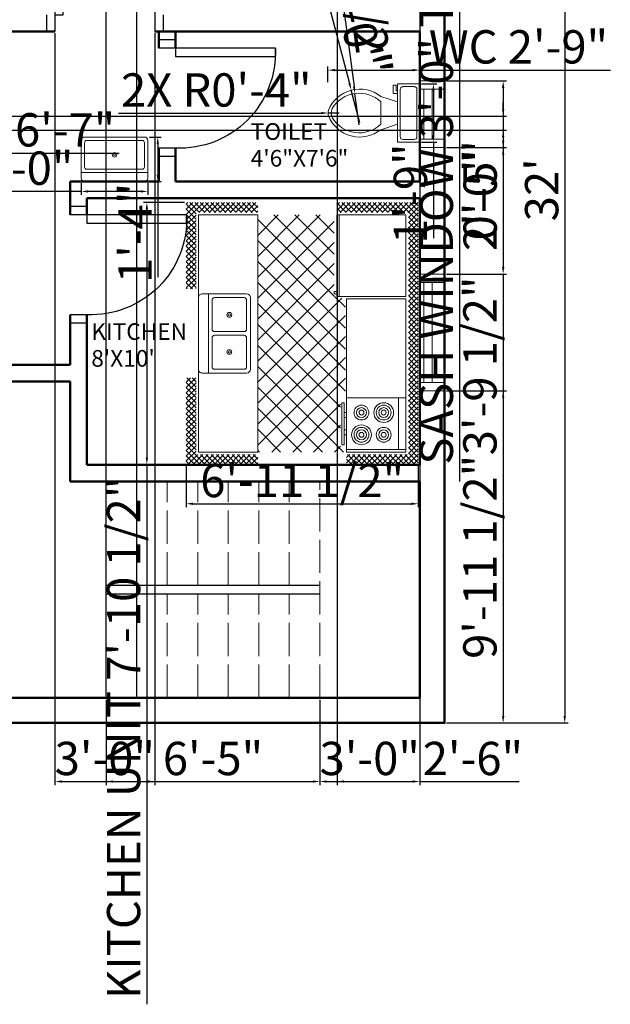
# Model space of a CAD drawing. Units: inches. Extents: x 3705 to 4206, y -1241 to -584.
# Tile 2 of 3: x 3921 to 4134, y -1241 to -886. Entities that reach past the tile are written whole.
import ezdxf

# ---------------------------------------------------------------- set-up
doc = ezdxf.new("R2010")
doc.units = ezdxf.units.IN
doc.linetypes.add('ACAD_ISO02W100', pattern=[15, 12, -3])
for name, color, linetype, lineweight in [('A-ANNO-DIMS', 2, 'Continuous', 18), ('A-AREA-IDEN', 7, 'Continuous', 25), ('A-DOOR', 3, 'Continuous', 25), ('A-FLOR-FIXT', 9, 'Continuous', 18), ('A-FLOR-STRS', 7, 'Continuous', 25), ('A-FLOR-STRS-HIDN', 8, 'ACAD_ISO02W100', 18), ('A-GLAZ', 4, 'Continuous', 18), ('A-WALL', 7, 'Continuous', 50)]:
    doc.layers.add(name, color=color, linetype=linetype, lineweight=lineweight)
doc.styles.get("Standard").update_dxf_attribs({"font": 'arial.ttf'})
doc.dimstyles.new('ISO-25', dxfattribs={"dimtxt": 12, "dimasz": 2.5, "dimexe": 1.25, "dimexo": 0.625, "dimtad": 1, "dimdec": 1, "dimlunit": 3, "dimtxsty": 'Standard', "dimcen": 2.5, "dimadec": 0, "dimazin": 0, "dimtfac": 1, "dimtdec": 1, "dimtmove": 0, "dimatfit": 3, "dimfxl": 1, "dimarcsym": 0})

# ---------------------------------------------------------------- blocks, each defined once
blk = doc.blocks.new('Toilet - top')
for p, q in [((9.5, -6), (9.5, -2)), ((-10, -8.5), (-8, -8.5)), ((-10, -9.5), (-10, -8.5)), ((-7, -9.5), (-10, -9.5)), ((-8, -8.5), (-8, -8)), ((-7, -8), (-7, -9.5)), ((-4, -8), (-6, -14)), ((4, -8), (6, -14)), ((4, -14), (-4, -14))]:
    blk.add_line(p, q)
blk.add_lwpolyline([(10.5, -8), (10.5, 0), (-10.5, 0), (-10.5, -8)], close=True)
for points in [[(-9.5, -2), (-9.5, -6)], [(8.5, -1), (-8.5, -1)], [(-8.5, -7), (8.5, -7)]]:
    blk.add_lwpolyline(points)
for centre, radius, start, end in [((-8.62, -1.88), 0.884, 81.8699, 188.1301), ((8.62, -1.88), 0.884, 351.8699, 98.1301), ((-8.62, -6.12), 0.884, 171.8699, 278.1301), ((8.62, -6.12), 0.884, 261.8699, 8.1301), ((3.52, -21.58), 12.17, 141.4691, 247.9714), ((4.2, -21.82), 11.33, 136.3677, 238.9468), ((-3.52, -21.58), 12.17, 292.0284, 38.5307), ((-4.2, -21.82), 11.33, 301.053, 43.6321), ((0, -27.88), 4, 245.7318, 294.2682), ((0, -29), 4, 254.8605, 285.1395)]:
    blk.add_arc(centre, radius, start, end)
blk = doc.blocks.new('Sink-single - 30 in top')
blk.add_line((-15, -3.999996), (15, -3.999996))
for points in [[(-13.5, 0), (13.5, 0)], [(-15, -18.499996), (-15, -1.5)], [(15, -1.5), (15, -18.499996)], [(-13.5, -17.499996), (-13.5, -6.499996)], [(-12.5, -5.499996), (12.5, -5.499996)], [(13.5, -6.499996), (13.5, -17.499996)], [(13.5, -19.999996), (-13.5, -19.999996)], [(12.5, -18.499996), (-12.5, -18.499996)]]:
    blk.add_lwpolyline(points)
for radius in [1, 0.5]:
    blk.add_circle((0, -11.999996), radius)
for centre, radius, start, end in [((-13.5, -1.5), 1.5, 90, 180), ((13.5, -1.5), 1.5, 0, 90), ((-12.5, -6.499996), 1, 90, 180), ((12.5, -6.499996), 1, 0, 90), ((-12.5, -17.499996), 1, 180, 270), ((12.5, -17.499996), 1, 270, 0), ((-13.5, -18.499996), 1.5, 180, 270), ((13.5, -18.499996), 1.5, 270, 0)]:
    blk.add_arc(centre, radius, start, end)
blk = doc.blocks.new('Kitchen Layout - 7 x 8 ft')
for p, q in [((-5, 81.32), (2.68, 89)), ((-5, 83.44), (0.56, 89)), ((-5, 85.56), (-1.56, 89)), ((-5, 87.68), (-3.68, 89)), ((-1, 84.97), (-5, 88.97)), ((1.09, 85), (-2.91, 89)), ((3.21, 85), (-0.79, 89)), ((0.81, 85), (4.81, 89)), ((5.34, 85), (1.34, 89)), ((2.93, 85), (6.93, 89)), ((7.46, 85), (3.46, 89)), ((5.05, 85), (9.05, 89)), ((9.58, 85), (5.58, 89)), ((7.17, 85), (11.17, 89)), ((11.7, 85), (7.7, 89)), ((9.29, 85), (13.29, 89)), ((13.82, 85), (9.82, 89)), ((11.41, 85), (15.41, 89)), ((15.94, 85), (11.94, 89)), ((13.53, 85), (17.53, 89)), ((18.06, 85), (14.06, 89)), ((15.65, 85), (19.65, 89)), ((20.18, 85), (16.18, 89)), ((17.78, 85), (21.78, 89)), ((22.31, 85), (18.31, 89)), ((19.9, 85), (23.9, 89)), ((24.43, 85), (20.43, 89)), ((22.02, 85), (26.02, 89)), ((26.55, 85), (22.55, 89)), ((24.14, 85), (28.14, 89)), ((28.67, 85), (24.67, 89)), ((26.26, 85), (30.26, 89)), ((30.79, 85), (26.79, 89)), ((28.38, 85), (32.38, 89)), ((32.91, 85), (28.91, 89)), ((30.5, 85), (34.5, 89)), ((35.03, 85), (31.03, 89)), ((32.63, 85), (36.63, 89)), ((37.16, 85), (33.16, 89)), ((34.75, 85), (38.75, 89)), ((39.28, 85), (35.28, 89)), ((36.87, 85), (40.87, 89)), ((41.4, 85), (37.4, 89)), ((38.99, 85), (42.99, 89)), ((43.52, 85), (39.52, 89)), ((41.11, 85), (45.11, 89)), ((45.64, 85), (41.64, 89)), ((43.23, 85), (47.23, 89)), ((47.76, 85), (43.76, 89)), ((45.35, 85), (49.35, 89)), ((49.88, 85), (45.88, 89)), ((47.47, 85), (51.47, 89)), ((52, 85), (48, 89)), ((49.6, 85), (53.6, 89)), ((54.13, 85), (50.13, 89)), ((51.72, 85), (55.72, 89)), ((56.25, 85), (52.25, 89)), ((53.84, 85), (57.84, 89)), ((58.37, 85), (54.37, 89)), ((55.96, 85), (59.96, 89)), ((60.49, 85), (56.49, 89)), ((58.08, 85), (62.08, 89)), ((62.61, 85), (58.61, 89)), ((60.2, 85), (64.2, 89)), ((64.73, 85), (60.73, 89)), ((62.32, 85), (66.32, 89)), ((66.85, 85), (62.85, 89)), ((64.45, 85), (68.45, 89)), ((68.97, 85), (64.97, 89)), ((66.57, 85), (70.57, 89)), ((71.1, 85), (67.1, 89)), ((68.69, 85), (72.69, 89)), ((73.22, 85), (69.22, 89)), ((70.81, 85), (74.81, 89)), ((75.34, 85), (71.34, 89)), ((72.93, 85), (76.93, 89)), ((77.46, 85), (73.46, 89)), ((75.05, 85), (79.05, 89)), ((79.58, 85), (75.58, 89)), ((77.17, 85), (81.17, 89)), ((81.7, 85), (77.7, 89)), ((79.29, 85), (83.29, 89)), ((83.82, 85), (79.82, 89)), ((81.42, 85), (85.42, 89)), ((85.95, 85), (81.95, 89)), ((83.54, 85), (87.54, 89)), ((88.07, 85), (84.07, 89)), ((85.66, 85), (89.66, 89)), ((90.19, 85), (86.19, 89)), ((87.78, 85), (91.78, 89)), ((92.31, 85), (88.31, 89)), ((89.9, 85), (93.9, 89)), ((94.43, 85), (90.43, 89)), ((92.02, 85), (96.02, 89)), ((96.55, 85), (92.55, 89)), ((94.14, 85), (98.14, 89)), ((101, 82.67), (94.67, 89)), ((96.27, 85), (100.27, 89)), ((101, 84.79), (96.79, 89)), ((101, 86.92), (98.92, 89)), ((-1, 82.85), (-5, 86.85)), ((-1, 80.73), (-5, 84.73)), ((34, 84), (96, 84)), ((34, 60), (34, 84)), ((96, 84), (96, 60)), ((97, 83.61), (101, 87.61)), ((97, 81.49), (101, 85.49)), ((101, 80.55), (97, 84.55)), ((-5, 79.19), (-1, 83.19)), ((-1, 78.61), (-5, 82.61)), ((-5, 77.07), (-1, 81.07)), ((-1, 76.49), (-5, 80.49)), ((74, 81), (95, 81)), ((97, 79.37), (101, 83.37)), ((101, 78.43), (97, 82.43)), ((97, 77.25), (101, 81.25)), ((101, 76.31), (97, 80.31)), ((-5, 74.95), (-1, 78.95)), ((-1, 74.36), (-5, 78.36)), ((-5, 72.83), (-1, 76.83)), ((-1, 72.24), (-5, 76.24)), ((97, 75.13), (101, 79.13)), ((101, 74.19), (97, 78.19)), ((97, 73.01), (101, 77.01)), ((101, 72.07), (97, 76.07)), ((-5, 70.71), (-1, 74.71)), ((-1, 70.12), (-5, 74.12)), ((-5, 68.59), (-1, 72.59)), ((-1, 68), (-5, 72)), ((97, 70.89), (101, 74.89)), ((101, 69.95), (97, 73.95)), ((97, 68.76), (101, 72.76)), ((101, 67.82), (97, 71.82)), ((-5, 66.47), (-1, 70.47)), ((-1, 65.88), (-5, 69.88)), ((-5, 64.35), (-1, 68.35)), ((-1, 63.76), (-5, 67.76)), ((97, 66.64), (101, 70.64)), ((101, 65.7), (97, 69.7)), ((97, 64.52), (101, 68.52)), ((-5, 62.22), (-1, 66.22)), ((-1, 61.64), (-5, 65.64)), ((-5, 60.1), (-1, 64.1)), ((101, 63.58), (97, 67.58)), ((97, 62.4), (101, 66.4)), ((101, 61.46), (97, 65.46)), ((97, 60.28), (101, 64.28)), ((-1, 59.52), (-5, 63.52)), ((-5, 57.98), (-1, 61.98)), ((-1, 57.39), (-5, 61.39)), ((-4.86, 56), (-1, 59.86)), ((96, 60), (34, 60)), ((80, 60), (80, 59)), ((82, 59), (82, 60)), ((87, 59), (87, 60)), ((89, 60), (89, 59)), ((100.34, 60), (97, 63.34)), ((98.22, 60), (97, 61.22)), ((98.84, 60), (101, 62.16)), ((100.96, 60), (101, 60.04)), ((-1.73, 56), (-5, 59.27)), ((-3.85, 56), (-5, 57.15)), ((-2.74, 56), (-1, 57.74)), ((0, 57), (33, 57)), ((10.4, 24), (45.9, 59.5)), ((18.88, 24), (54.38, 59.5)), ((27.37, 24), (62.87, 59.5)), ((31, 55), (31, 56)), ((32, 56), (32, 55)), ((33.03, 55.11), (37.41, 59.5)), ((67.71, 24), (33.68, 58.04)), ((35.85, 24), (71.35, 59.5)), ((76.2, 24), (40.7, 59.5)), ((44.34, 24), (77.84, 57.5)), ((84.68, 24), (49.18, 59.5)), ((52.82, 24), (86.32, 57.5)), ((93.17, 24), (57.67, 59.5)), ((61.31, 24), (96, 58.69)), ((96, 29.65), (66.15, 59.5)), ((96, 38.14), (76.64, 57.5)), ((96, 46.63), (85.13, 57.5)), ((96, 55.11), (93.57, 57.54)), ((0, 30.57), (24.43, 55)), ((0, 39.06), (15.94, 55)), ((0, 47.54), (7.46, 55)), ((1.91, 24), (32.91, 55)), ((33.77, 24), (2.77, 55)), ((42.26, 24), (11.26, 55)), ((50.74, 24), (19.74, 55)), ((59.23, 24), (28.23, 55)), ((32, 55), (31, 55)), ((25.29, 24), (0, 49.29)), ((69.79, 24), (96, 50.21)), ((16.8, 24), (0, 40.8)), ((78.28, 24), (96, 41.72)), ((8.32, 24), (0, 32.32)), ((86.76, 24), (96, 33.24)), ((-5, 21.92), (-2.92, 24)), ((-1, 21.33), (-3.67, 24)), ((-1, 23.45), (-1.55, 24)), ((0, 24), (96, 24)), ((0, 0), (0, 24)), ((95.25, 24), (96, 24.75)), ((96, 24), (96, 0)), ((97, 22.1), (98.9, 24)), ((97, 19.97), (101, 23.97)), ((101, 21.16), (98.16, 24)), ((101, 23.28), (100.28, 24)), ((-5, 19.8), (-1, 23.8)), ((-1, 19.21), (-5, 23.21)), ((-5, 17.68), (-1, 21.68)), ((-1, 17.09), (-5, 21.09)), ((101, 19.03), (97, 23.03)), ((97, 17.85), (101, 21.85)), ((101, 16.91), (97, 20.91)), ((-5, 15.55), (-1, 19.55)), ((-1, 14.97), (-5, 18.97)), ((-5, 13.43), (-1, 17.43)), ((-1, 12.85), (-5, 16.85)), ((47.25, 6.5), (47.25, 18.5)), ((48.75, 18.5), (48.75, 6.5)), ((97, 15.73), (101, 19.73)), ((101, 14.79), (97, 18.79)), ((97, 13.61), (101, 17.61)), ((101, 12.67), (97, 16.67)), ((-5, 11.31), (-1, 15.31)), ((-1, 10.73), (-5, 14.73)), ((-5, 9.19), (-1, 13.19)), ((-1, 8.6), (-5, 12.6)), ((97, 11.49), (101, 15.49)), ((101, 10.55), (97, 14.55)), ((97, 9.37), (101, 13.37)), ((101, 8.43), (97, 12.43)), ((-5, 7.07), (-1, 11.07)), ((-1, 6.48), (-5, 10.48)), ((-5, 4.95), (-1, 8.95)), ((-1, 4.36), (-5, 8.36)), ((97, 7.25), (101, 11.25)), ((101, 6.31), (97, 10.31)), ((97, 5.12), (101, 9.12)), ((101, 4.18), (97, 8.18)), ((-5, 2.83), (-1, 6.83)), ((-1, 2.24), (-5, 6.24)), ((-5, 0.71), (-1, 4.71)), ((-1, 0.12), (-5, 4.12)), ((64, 4), (32, 4)), ((97, 3), (101, 7)), ((101, 2.06), (97, 6.06)), ((97, 0.88), (101, 4.88)), ((-5, -1.42), (-1, 2.58)), ((2, -5), (-5, 2)), ((-5, -3.54), (-1, 0.46)), ((96, 0), (0, 0)), ((93.24, -5), (101, 2.76)), ((95.36, -5), (101, 0.64)), ((101, -0.06), (97, 3.94)), ((101, -2.18), (97, 1.82)), ((-0.12, -5), (-5, -0.12)), ((-2.25, -5), (-5, -2.25)), ((-4.34, -5), (-0.34, -1)), ((-2.22, -5), (1.78, -1)), ((-0.1, -5), (3.9, -1)), ((4.12, -5), (0.12, -1)), ((2.02, -5), (6.02, -1)), ((6.24, -5), (2.24, -1)), ((4.14, -5), (8.14, -1)), ((8.36, -5), (4.36, -1)), ((6.27, -5), (10.27, -1)), ((10.48, -5), (6.48, -1)), ((8.39, -5), (12.39, -1)), ((12.6, -5), (8.6, -1)), ((10.51, -5), (14.51, -1)), ((14.73, -5), (10.73, -1)), ((12.63, -5), (16.63, -1)), ((16.85, -5), (12.85, -1)), ((14.75, -5), (18.75, -1)), ((18.97, -5), (14.97, -1)), ((16.87, -5), (20.87, -1)), ((21.09, -5), (17.09, -1)), ((18.99, -5), (22.99, -1)), ((23.21, -5), (19.21, -1)), ((21.11, -5), (25.11, -1)), ((25.33, -5), (21.33, -1)), ((23.24, -5), (27.24, -1)), ((27.45, -5), (23.45, -1)), ((25.36, -5), (29.36, -1)), ((29.57, -5), (25.57, -1)), ((27.48, -5), (30, -2.48)), ((30, -3.3), (27.7, -1)), ((30, -1.18), (29.82, -1)), ((66, -2.54), (67.54, -1)), ((66, -4.66), (69.66, -1)), ((69.88, -5), (66, -1.12)), ((67.76, -5), (66, -3.24)), ((67.78, -5), (71.78, -1)), ((72, -5), (68, -1)), ((69.9, -5), (73.9, -1)), ((74.12, -5), (70.12, -1)), ((72.03, -5), (76.03, -1)), ((76.24, -5), (72.24, -1)), ((74.15, -5), (78.15, -1)), ((78.36, -5), (74.36, -1)), ((76.27, -5), (80.27, -1)), ((80.49, -5), (76.49, -1)), ((78.39, -5), (82.39, -1)), ((82.61, -5), (78.61, -1)), ((80.51, -5), (84.51, -1)), ((84.73, -5), (80.73, -1)), ((82.63, -5), (86.63, -1)), ((86.85, -5), (82.85, -1)), ((84.75, -5), (88.75, -1)), ((88.97, -5), (84.97, -1)), ((86.88, -5), (90.88, -1)), ((91.09, -5), (87.09, -1)), ((89, -5), (93, -1)), ((93.21, -5), (89.21, -1)), ((91.12, -5), (95.12, -1)), ((95.34, -5), (91.34, -1)), ((97.46, -5), (93.46, -1)), ((99.58, -5), (95.58, -1)), ((101, -4.3), (97, -0.3)), ((97.48, -5), (101, -1.48)), ((99.6, -5), (101, -3.6)), ((-4.37, -5), (-5, -4.37)), ((29.6, -5), (30, -4.6))]:
    blk.add_line(p, q)
for points in [[(0, 56), (0, 84), (33, 84), (33, 56)], [(74, 60), (74, 84), (95, 84), (95, 60)], [(76, 58), (76, 59), (93, 59), (93, 58)]]:
    blk.add_lwpolyline(points, close=True)
for points in [[(33.5, 21), (62.5, 21)], [(32, 1.5), (32, 19.5)], [(33.5, 6.5), (33.5, 18.5)], [(34.5, 19.5), (46.25, 19.5)], [(49.75, 19.5), (61.5, 19.5)], [(62.5, 18.5), (62.5, 6.5)], [(64, 19.5), (64, 1.5)], [(46.25, 5.5), (34.5, 5.5)], [(61.5, 5.5), (49.75, 5.5)], [(62.5, 0), (33.5, 0)]]:
    blk.add_lwpolyline(points)
for centre, radius in [((80, 75), 4), ((80, 75), 3), ((80, 75), 2), ((80, 75), 1), ((89, 75), 3), ((89, 75), 2), ((89, 75), 1), ((80, 66), 3), ((80, 66), 2), ((89, 66), 4), ((89, 66), 3), ((89, 66), 2), ((80, 66), 1), ((89, 66), 1), ((40.5, 12.5), 1), ((40.5, 12.5), 0.5), ((55.5, 12.5), 1), ((55.5, 12.5), 0.5)]:
    blk.add_circle(centre, radius)
for centre, radius, start, end in [((33.5, 19.5), 1.5, 90, 180), ((62.5, 19.5), 1.5, 0, 90), ((34.5, 18.5), 1, 90, 180), ((46.25, 18.5), 1, 0, 90), ((49.75, 18.5), 1, 90, 180), ((61.5, 18.5), 1, 0, 90), ((34.5, 6.5), 1, 180, 270), ((46.25, 6.5), 1, 270, 0), ((49.75, 6.5), 1, 180, 270), ((61.5, 6.5), 1, 270, 0), ((33.5, 1.5), 1.5, 180, 270), ((62.5, 1.5), 1.5, 270, 0)]:
    blk.add_arc(centre, radius, start, end)
blk = doc.blocks.new('*D12')
at = {"layer": 'A-ANNO-DIMS', "color": 0, "lineweight": -2, "transparency": 16777216}
for p, q in [((4074.7, -755.75), (4118.62, -755.75)), ((4117.37, -758.25), (4117.37, -1137.25)), ((4074.7, -1139.75), (4118.62, -1139.75))]:
    blk.add_line(p, q, dxfattribs=at)
at = {"layer": 'A-ANNO-DIMS', "color": 0, "transparency": 16777216}
for points in [[(4116.95, -758.25), (4117.78, -758.25), (4117.37, -755.75)], [(4116.95, -1137.25), (4117.78, -1137.25), (4117.37, -1139.75)]]:
    blk.add_solid(points, dxfattribs=at)
at = {"layer": 'Defpoints', "color": 0, "transparency": 16777216}
for p in [(4074.08, -755.75), (4074.08, -1139.75), (4117.37, -1139.75)]:
    blk.add_point(p, dxfattribs=at)
at = {"layer": 'A-ANNO-DIMS', "color": 0, "transparency": 16777216, "insert": (4110.61, -947.75), "char_height": 12, "attachment_point": 5, "rotation": 90}
blk.add_mtext("32'", dxfattribs=at)
blk = doc.blocks.new('DOOR-SINGLE-36IN')
for p, q in [((0, 6), (0, 0)), ((3, 6), (3, 0)), ((39, 6), (39, 0)), ((42, 6), (42, 0))]:
    blk.add_line(p, q)
blk.add_lwpolyline([(39, 6), (36, 6), (36, 42), (39, 42)], close=True)
blk.add_arc((37.5, 7.5), 34.53, 87.5104, 182.4896)
blk = doc.blocks.new('WIN-SASH-36IN')
for p, q in [((0, 9), (0, 0)), ((36, 0), (36, 9)), ((0, 4.5), (36, 4.5)), ((0, 1.5), (36, 1.5)), ((0, 1.5), (36, 1.5))]:
    blk.add_line(p, q)
blk = doc.blocks.new('*D15')
at = {"layer": 'A-ANNO-DIMS', "color": 0, "lineweight": -2, "transparency": 16777216}
for p, q in [((4074.7, -811.42), (4080.73, -811.42)), ((4079.48, -813.92), (4079.48, -844.92)), ((4074.7, -847.42), (4080.73, -847.42)), ((4079.48, -847.42), (4079.48, -1052.78))]:
    blk.add_line(p, q, dxfattribs=at)
at = {"layer": 'A-ANNO-DIMS', "color": 0, "transparency": 16777216}
for points in [[(4079.06, -813.92), (4079.9, -813.92), (4079.48, -811.42)], [(4079.06, -844.92), (4079.9, -844.92), (4079.48, -847.42)]]:
    blk.add_solid(points, dxfattribs=at)
at = {"layer": 'Defpoints', "color": 0, "transparency": 16777216}
for p in [(4074.08, -811.42), (4074.08, -847.42), (4079.48, -847.42)]:
    blk.add_point(p, dxfattribs=at)
at = {"layer": 'A-ANNO-DIMS', "color": 0, "transparency": 16777216, "insert": (4072.64, -951.35), "char_height": 12, "attachment_point": 5, "rotation": 90}
blk.add_mtext('SASH WINDOW 3\'-0" TYP.', dxfattribs=at)
blk = doc.blocks.new('*D25')
at = {"layer": 'A-ANNO-DIMS', "color": 0, "lineweight": -2, "transparency": 16777216}
for p, q in [((3791.85, -923.33), (3791.85, -935.8)), ((3870.81, -923.33), (3870.81, -935.8)), ((3794.35, -934.55), (3868.31, -934.55)), ((3870.81, -934.55), (3956.7, -934.55))]:
    blk.add_line(p, q, dxfattribs=at)
at = {"layer": 'A-ANNO-DIMS', "color": 0, "transparency": 16777216}
for points in [[(3794.35, -934.13), (3794.35, -934.97), (3791.85, -934.55)], [(3868.31, -934.13), (3868.31, -934.97), (3870.81, -934.55)]]:
    blk.add_solid(points, dxfattribs=at)
at = {"layer": 'Defpoints', "color": 0, "transparency": 16777216}
for p in [(3791.85, -922.71), (3870.81, -922.71), (3870.81, -934.55)]:
    blk.add_point(p, dxfattribs=at)
at = {"layer": 'A-ANNO-DIMS', "color": 0, "transparency": 16777216, "insert": (3915, -927.72), "char_height": 12, "attachment_point": 5}
blk.add_mtext('SOFA 6\'-7"', dxfattribs=at)
blk = doc.blocks.new('*D29')
at = {"layer": 'A-ANNO-DIMS', "color": 0, "lineweight": -2, "transparency": 16777216}
for p, q in [((4032.03, -908.99), (4032.03, -903.41)), ((4065.08, -908.99), (4065.08, -903.41)), ((4034.53, -904.66), (4062.58, -904.66)), ((4065.08, -904.66), (4133.81, -904.66))]:
    blk.add_line(p, q, dxfattribs=at)
at = {"layer": 'A-ANNO-DIMS', "color": 0, "transparency": 16777216}
for points in [[(4034.53, -904.24), (4034.53, -905.07), (4032.03, -904.66)], [(4062.58, -904.24), (4062.58, -905.07), (4065.08, -904.66)]]:
    blk.add_solid(points, dxfattribs=at)
at = {"layer": 'Defpoints', "color": 0, "transparency": 16777216}
for p in [(4065.08, -904.66), (4032.03, -909.61), (4065.08, -909.61)]:
    blk.add_point(p, dxfattribs=at)
at = {"layer": 'A-ANNO-DIMS', "color": 0, "transparency": 16777216, "insert": (4100.69, -897.83), "char_height": 12, "attachment_point": 5}
blk.add_mtext('WC 2\'-9"', dxfattribs=at)
blk = doc.blocks.new('*D30')
at = {"layer": 'A-ANNO-DIMS', "color": 0, "lineweight": -2, "transparency": 16777216}
for p, q in [((4065.7, -909.61), (4071.29, -909.61)), ((4070.04, -912.11), (4070.04, -928.11)), ((4065.7, -930.61), (4071.29, -930.61)), ((4070.04, -930.61), (4070.04, -965.13))]:
    blk.add_line(p, q, dxfattribs=at)
at = {"layer": 'A-ANNO-DIMS', "color": 0, "transparency": 16777216}
for points in [[(4069.62, -912.11), (4070.45, -912.11), (4070.04, -909.61)], [(4069.62, -928.11), (4070.45, -928.11), (4070.04, -930.61)]]:
    blk.add_solid(points, dxfattribs=at)
at = {"layer": 'Defpoints', "color": 0, "transparency": 16777216}
for p in [(4065.08, -909.61), (4065.08, -930.61), (4070.04, -930.61)]:
    blk.add_point(p, dxfattribs=at)
at = {"layer": 'A-ANNO-DIMS', "color": 0, "transparency": 16777216, "insert": (4063.28, -949.12), "char_height": 12, "attachment_point": 5, "rotation": 90}
blk.add_mtext('1\'-9"', dxfattribs=at)
blk = doc.blocks.new('*D31')
at = {"layer": 'A-ANNO-DIMS', "color": 0, "lineweight": -2, "transparency": 16777216}
for p, q in [((3943.08, -945.37), (3943.08, -949.6)), ((3967.08, -945.37), (3967.08, -949.6)), ((3943.08, -948.35), (3853, -948.35)), ((3964.58, -948.35), (3945.58, -948.35))]:
    blk.add_line(p, q, dxfattribs=at)
at = {"layer": 'A-ANNO-DIMS', "color": 0, "transparency": 16777216}
for points in [[(3945.58, -947.93), (3945.58, -948.76), (3943.08, -948.35)], [(3964.58, -947.93), (3964.58, -948.76), (3967.08, -948.35)]]:
    blk.add_solid(points, dxfattribs=at)
at = {"layer": 'Defpoints', "color": 0, "transparency": 16777216}
for p in [(3943.08, -944.75), (3967.08, -944.75), (3943.08, -948.35)]:
    blk.add_point(p, dxfattribs=at)
at = {"layer": 'A-ANNO-DIMS', "color": 0, "transparency": 16777216, "insert": (3896.79, -941.52), "char_height": 12, "attachment_point": 5}
blk.add_mtext('BASIN 2\'-0"', dxfattribs=at)
blk = doc.blocks.new('*D32')
at = {"layer": 'A-ANNO-DIMS', "color": 0, "lineweight": -2, "transparency": 16777216}
for p, q in [((3967.7, -928.75), (3971.93, -928.75)), ((3970.68, -931.25), (3970.68, -942.25)), ((3967.7, -944.75), (3971.93, -944.75)), ((3970.68, -944.75), (3970.68, -979.27))]:
    blk.add_line(p, q, dxfattribs=at)
at = {"layer": 'A-ANNO-DIMS', "color": 0, "transparency": 16777216}
for points in [[(3970.26, -931.25), (3971.1, -931.25), (3970.68, -928.75)], [(3970.26, -942.25), (3971.1, -942.25), (3970.68, -944.75)]]:
    blk.add_solid(points, dxfattribs=at)
at = {"layer": 'Defpoints', "color": 0, "transparency": 16777216}
for p in [(3967.08, -928.75), (3967.08, -944.75), (3970.68, -944.75)]:
    blk.add_point(p, dxfattribs=at)
at = {"layer": 'A-ANNO-DIMS', "color": 0, "transparency": 16777216, "insert": (3964.03, -963.26), "char_height": 12, "attachment_point": 5, "rotation": 90}
blk.add_mtext('1\'-4"', dxfattribs=at)
blk = doc.blocks.new('*D33')
at = {"layer": 'A-ANNO-DIMS', "color": 0, "lineweight": -2, "transparency": 16777216}
for p, q in [((3980.27, -952.31), (3965.49, -952.31)), ((3966.74, -954.81), (3966.74, -1044.17)), ((3980.27, -1046.67), (3965.49, -1046.67)), ((3966.74, -1046.67), (3966.74, -1241.08))]:
    blk.add_line(p, q, dxfattribs=at)
at = {"layer": 'A-ANNO-DIMS', "color": 0, "transparency": 16777216}
for points in [[(3966.32, -954.81), (3967.16, -954.81), (3966.74, -952.31)], [(3966.32, -1044.17), (3967.16, -1044.17), (3966.74, -1046.67)]]:
    blk.add_solid(points, dxfattribs=at)
at = {"layer": 'Defpoints', "color": 0, "transparency": 16777216}
for p in [(3980.9, -952.31), (3966.74, -1046.67), (3980.9, -1046.67)]:
    blk.add_point(p, dxfattribs=at)
at = {"layer": 'A-ANNO-DIMS', "color": 0, "transparency": 16777216, "insert": (3959.91, -1145.12), "char_height": 12, "attachment_point": 5, "rotation": 90}
blk.add_mtext('KITCHEN UNIT 7\'-10 1/2"', dxfattribs=at)
blk = doc.blocks.new('*D34')
at = {"layer": 'A-ANNO-DIMS', "color": 0, "lineweight": -2, "transparency": 16777216}
for p, q in [((3980.9, -1047.29), (3980.9, -1062.07)), ((4064.57, -1047.29), (4064.57, -1062.07)), ((3983.4, -1060.82), (4062.07, -1060.82))]:
    blk.add_line(p, q, dxfattribs=at)
at = {"layer": 'A-ANNO-DIMS', "color": 0, "transparency": 16777216}
for points in [[(3983.4, -1060.4), (3983.4, -1061.24), (3980.9, -1060.82)], [(4062.07, -1060.4), (4062.07, -1061.24), (4064.57, -1060.82)]]:
    blk.add_solid(points, dxfattribs=at)
at = {"layer": 'Defpoints', "color": 0, "transparency": 16777216}
for p in [(3980.9, -1046.67), (4064.57, -1046.67), (4064.57, -1060.82)]:
    blk.add_point(p, dxfattribs=at)
at = {"layer": 'A-ANNO-DIMS', "color": 0, "transparency": 16777216, "insert": (4022.73, -1053.99), "char_height": 12, "attachment_point": 5}
blk.add_mtext('6\'-11 1/2"', dxfattribs=at)
blk = doc.blocks.new('*D40')
at = {"layer": 'A-ANNO-DIMS', "color": 0, "lineweight": -2, "transparency": 16777216}
for p, q in [((4074.7, -1020.11), (4096.43, -1020.11)), ((4095.18, -1022.61), (4095.18, -1137.25)), ((4074.7, -1139.75), (4096.43, -1139.75))]:
    blk.add_line(p, q, dxfattribs=at)
at = {"layer": 'A-ANNO-DIMS', "color": 0, "transparency": 16777216}
for points in [[(4094.76, -1022.61), (4095.6, -1022.61), (4095.18, -1020.11)], [(4094.76, -1137.25), (4095.6, -1137.25), (4095.18, -1139.75)]]:
    blk.add_solid(points, dxfattribs=at)
at = {"layer": 'Defpoints', "color": 0, "transparency": 16777216}
for p in [(4074.08, -1020.11), (4074.08, -1139.75), (4095.18, -1139.75)]:
    blk.add_point(p, dxfattribs=at)
at = {"layer": 'A-ANNO-DIMS', "color": 0, "transparency": 16777216, "insert": (4088.35, -1079.93), "char_height": 12, "attachment_point": 5, "rotation": 90}
blk.add_mtext('9\'-11 1/2"', dxfattribs=at)
blk = doc.blocks.new('*D41')
at = {"layer": 'A-ANNO-DIMS', "color": 0, "lineweight": -2, "transparency": 16777216}
for p, q in [((4074.7, -932.56), (4096.43, -932.56)), ((4095.18, -935.06), (4095.18, -975.61)), ((4074.7, -978.11), (4096.43, -978.11)), ((4095.18, -978.11), (4095.18, -1041.72))]:
    blk.add_line(p, q, dxfattribs=at)
at = {"layer": 'A-ANNO-DIMS', "color": 0, "transparency": 16777216}
for points in [[(4094.76, -935.06), (4095.6, -935.06), (4095.18, -932.56)], [(4094.76, -975.61), (4095.6, -975.61), (4095.18, -978.11)]]:
    blk.add_solid(points, dxfattribs=at)
at = {"layer": 'Defpoints', "color": 0, "transparency": 16777216}
for p in [(4074.08, -932.56), (4074.08, -978.11), (4095.18, -978.11)]:
    blk.add_point(p, dxfattribs=at)
at = {"layer": 'A-ANNO-DIMS', "color": 0, "transparency": 16777216, "insert": (4088.35, -1011.17), "char_height": 12, "attachment_point": 5, "rotation": 90}
blk.add_mtext('3\'-9 1/2"', dxfattribs=at)
blk = doc.blocks.new('*D42')
at = {"layer": 'A-ANNO-DIMS', "color": 0, "lineweight": -2, "transparency": 16777216}
for p, q in [((4074.7, -908.56), (4096.43, -908.56)), ((4095.18, -911.06), (4095.18, -930.06)), ((4074.7, -932.56), (4096.43, -932.56)), ((4095.18, -932.56), (4095.18, -968.41))]:
    blk.add_line(p, q, dxfattribs=at)
at = {"layer": 'A-ANNO-DIMS', "color": 0, "transparency": 16777216}
for points in [[(4094.76, -911.06), (4095.6, -911.06), (4095.18, -908.56)], [(4094.76, -930.06), (4095.6, -930.06), (4095.18, -932.56)]]:
    blk.add_solid(points, dxfattribs=at)
at = {"layer": 'Defpoints', "color": 0, "transparency": 16777216}
for p in [(4074.08, -908.56), (4074.08, -932.56), (4095.18, -932.56)]:
    blk.add_point(p, dxfattribs=at)
at = {"layer": 'A-ANNO-DIMS', "color": 0, "transparency": 16777216, "insert": (4088.43, -951.74), "char_height": 12, "attachment_point": 5, "rotation": 90}
blk.add_mtext('2\'-0"', dxfattribs=at)
blk = doc.blocks.new('*D45')
at = {"layer": 'A-ANNO-DIMS', "color": 0, "lineweight": -2, "transparency": 16777216}
for p, q in [((3952.08, -1131.37), (3952.08, -1162.1)), ((4029.08, -1131.37), (4029.08, -1162.1)), ((3954.58, -1160.85), (4026.58, -1160.85))]:
    blk.add_line(p, q, dxfattribs=at)
at = {"layer": 'A-ANNO-DIMS', "color": 0, "transparency": 16777216}
for points in [[(3954.58, -1160.43), (3954.58, -1161.26), (3952.08, -1160.85)], [(4026.58, -1160.43), (4026.58, -1161.26), (4029.08, -1160.85)]]:
    blk.add_solid(points, dxfattribs=at)
at = {"layer": 'Defpoints', "color": 0, "transparency": 16777216}
for p in [(3952.08, -1130.75), (4029.08, -1130.75), (4029.08, -1160.85)]:
    blk.add_point(p, dxfattribs=at)
at = {"layer": 'A-ANNO-DIMS', "color": 0, "transparency": 16777216, "insert": (3990.58, -1154.1), "char_height": 12, "attachment_point": 5}
blk.add_mtext('6\'-5"', dxfattribs=at)
blk = doc.blocks.new('*D46')
at = {"layer": 'A-ANNO-DIMS', "color": 0, "lineweight": -2, "transparency": 16777216}
for p, q in [((4029.08, -1131.37), (4029.08, -1162.1)), ((4065.08, -1131.37), (4065.08, -1162.1)), ((4031.58, -1160.85), (4062.58, -1160.85))]:
    blk.add_line(p, q, dxfattribs=at)
at = {"layer": 'A-ANNO-DIMS', "color": 0, "transparency": 16777216}
for points in [[(4031.58, -1160.43), (4031.58, -1161.26), (4029.08, -1160.85)], [(4062.58, -1160.43), (4062.58, -1161.26), (4065.08, -1160.85)]]:
    blk.add_solid(points, dxfattribs=at)
at = {"layer": 'Defpoints', "color": 0, "transparency": 16777216}
for p in [(4029.08, -1130.75), (4065.08, -1130.75), (4065.08, -1160.85)]:
    blk.add_point(p, dxfattribs=at)
at = {"layer": 'A-ANNO-DIMS', "color": 0, "transparency": 16777216, "insert": (4047.08, -1154.09), "char_height": 12, "attachment_point": 5}
blk.add_mtext('3\'-0"', dxfattribs=at)
blk = doc.blocks.new('*D51')
at = {"layer": 'A-ANNO-DIMS', "color": 0, "lineweight": -2, "transparency": 16777216}
for p, q in [((3933.58, -891.37), (3933.58, -1162.1)), ((3969.58, -891.37), (3969.58, -1162.1)), ((3936.08, -1160.85), (3967.08, -1160.85))]:
    blk.add_line(p, q, dxfattribs=at)
at = {"layer": 'A-ANNO-DIMS', "color": 0, "transparency": 16777216}
for points in [[(3936.08, -1160.43), (3936.08, -1161.26), (3933.58, -1160.85)], [(3967.08, -1160.43), (3967.08, -1161.26), (3969.58, -1160.85)]]:
    blk.add_solid(points, dxfattribs=at)
at = {"layer": 'Defpoints', "color": 0, "transparency": 16777216}
for p in [(3933.58, -890.75), (3969.58, -890.75), (3969.58, -1160.85)]:
    blk.add_point(p, dxfattribs=at)
at = {"layer": 'A-ANNO-DIMS', "color": 0, "transparency": 16777216, "insert": (3951.58, -1154.09), "char_height": 12, "attachment_point": 5}
blk.add_mtext('3\'-0"', dxfattribs=at)
blk = doc.blocks.new('*D53')
at = {"layer": 'A-ANNO-DIMS', "color": 0, "lineweight": -2, "transparency": 16777216}
for p, q in [((3952.08, -1130.12), (3952.08, -733.4)), ((3963.08, -1130.12), (3963.08, -733.4)), ((3954.58, -734.65), (3960.58, -734.65)), ((3963.08, -734.65), (4008.05, -734.65))]:
    blk.add_line(p, q, dxfattribs=at)
at = {"layer": 'A-ANNO-DIMS', "color": 0, "transparency": 16777216}
for points in [[(3954.58, -734.23), (3954.58, -735.06), (3952.08, -734.65)], [(3960.58, -734.23), (3960.58, -735.06), (3963.08, -734.65)]]:
    blk.add_solid(points, dxfattribs=at)
at = {"layer": 'Defpoints', "color": 0, "transparency": 16777216}
for p in [(3963.08, -734.65), (3952.08, -1130.75), (3963.08, -1130.75)]:
    blk.add_point(p, dxfattribs=at)
at = {"layer": 'A-ANNO-DIMS', "color": 0, "transparency": 16777216, "insert": (3986.82, -727.9), "char_height": 12, "attachment_point": 5}
blk.add_mtext('0\'-11"', dxfattribs=at)
blk = doc.blocks.new('*D55')
at = {"layer": 'A-ANNO-DIMS', "color": 0, "lineweight": -2, "transparency": 16777216}
for p, q in [((4035.32, -845.43), (4035.32, -1162.1)), ((4065.08, -851.05), (4065.08, -1162.1)), ((4037.82, -1160.85), (4062.58, -1160.85)), ((4065.08, -1160.85), (4100.93, -1160.85))]:
    blk.add_line(p, q, dxfattribs=at)
at = {"layer": 'A-ANNO-DIMS', "color": 0, "transparency": 16777216}
for points in [[(4037.82, -1160.43), (4037.82, -1161.26), (4035.32, -1160.85)], [(4062.58, -1160.43), (4062.58, -1161.26), (4065.08, -1160.85)]]:
    blk.add_solid(points, dxfattribs=at)
at = {"layer": 'Defpoints', "color": 0, "transparency": 16777216}
for p in [(4035.32, -844.8), (4065.08, -850.42), (4065.08, -1160.85)]:
    blk.add_point(p, dxfattribs=at)
at = {"layer": 'A-ANNO-DIMS', "color": 0, "transparency": 16777216, "insert": (4084.26, -1154.1), "char_height": 12, "attachment_point": 5}
blk.add_mtext('2\'-6"', dxfattribs=at)
blk = doc.blocks.new('*D59')
at = {"layer": 'A-ANNO-DIMS', "color": 0, "lineweight": -2, "transparency": 16777216}
for p, q in [((4095.18, -918.74), (4095.18, -916.24)), ((3865.79, -921.24), (4096.43, -921.24)), ((4095.18, -921.24), (4095.18, -926.33)), ((3837.22, -926.33), (4096.43, -926.33)), ((4095.18, -928.83), (4095.18, -964.48))]:
    blk.add_line(p, q, dxfattribs=at)
at = {"layer": 'A-ANNO-DIMS', "color": 0, "transparency": 16777216}
for points in [[(4094.76, -918.74), (4095.6, -918.74), (4095.18, -921.24)], [(4094.76, -928.83), (4095.6, -928.83), (4095.18, -926.33)]]:
    blk.add_solid(points, dxfattribs=at)
at = {"layer": 'Defpoints', "color": 0, "transparency": 16777216}
for p in [(3865.17, -921.24), (3836.59, -926.33), (4095.18, -926.33)]:
    blk.add_point(p, dxfattribs=at)
at = {"layer": 'A-ANNO-DIMS', "color": 0, "transparency": 16777216, "insert": (4088.43, -947.91), "char_height": 12, "attachment_point": 5, "rotation": 90}
blk.add_mtext('0\'-5"', dxfattribs=at)
blk = doc.blocks.new('*D66')
at = {"layer": 'A-ANNO-DIMS', "color": 0, "lineweight": -2, "transparency": 16777216}
for p, q in [((4021.19, -838.72), (4039.77, -909.45)), ((4043.5, -923.63), (4040.41, -911.86))]:
    blk.add_line(p, q, dxfattribs=at)
at = {"layer": 'A-ANNO-DIMS', "color": 0, "transparency": 16777216}
blk.add_solid([(4040.17, -909.34), (4039.37, -909.55), (4040.41, -911.86)], dxfattribs=at)
at = {"layer": 'Defpoints', "color": 0, "transparency": 16777216}
for p in [(4040.41, -911.86), (4043.5, -923.63)]:
    blk.add_point(p, dxfattribs=at)
at = {"layer": 'A-ANNO-DIMS', "color": 0, "transparency": 16777216, "insert": (4036.7, -871.16), "char_height": 12, "attachment_point": 5, "rotation": 284.7176}
blk.add_mtext('2X R1\'-0"', dxfattribs=at)
blk = doc.blocks.new('*D67')
at = {"layer": 'A-ANNO-DIMS', "color": 0, "lineweight": -2, "transparency": 16777216}
for p, q in [((4026.71, -801.19), (4041.42, -910.61)), ((4043.26, -924.31), (4041.75, -913.09))]:
    blk.add_line(p, q, dxfattribs=at)
at = {"layer": 'A-ANNO-DIMS', "color": 0, "transparency": 16777216}
blk.add_solid([(4041.83, -910.55), (4041.01, -910.66), (4041.75, -913.09)], dxfattribs=at)
at = {"layer": 'Defpoints', "color": 0, "transparency": 16777216}
for p in [(4041.75, -913.09), (4043.26, -924.31)]:
    blk.add_point(p, dxfattribs=at)
at = {"layer": 'A-ANNO-DIMS', "color": 0, "transparency": 16777216, "insert": (4040.66, -853.75), "char_height": 12, "attachment_point": 5, "rotation": 277.6579}
blk.add_mtext('2X R0\'-11 1/2"', dxfattribs=at)
blk = doc.blocks.new('*D68')
at = {"layer": 'A-ANNO-DIMS', "color": 0, "lineweight": -2, "transparency": 16777216}
for p, q in [((3956.46, -920.11), (4029.58, -920.11)), ((4036.08, -920.11), (4032.08, -920.11))]:
    blk.add_line(p, q, dxfattribs=at)
at = {"layer": 'A-ANNO-DIMS', "color": 0, "transparency": 16777216}
blk.add_solid([(4029.58, -919.7), (4029.58, -920.53), (4032.08, -920.11)], dxfattribs=at)
at = {"layer": 'Defpoints', "color": 0, "transparency": 16777216}
for p in [(4032.08, -920.11), (4036.08, -920.11)]:
    blk.add_point(p, dxfattribs=at)
at = {"layer": 'A-ANNO-DIMS', "color": 0, "transparency": 16777216, "insert": (3991.77, -913.36), "char_height": 12, "attachment_point": 5, "rotation": 359.9938}
blk.add_mtext('2X R0\'-4"', dxfattribs=at)

msp = doc.modelspace()

# ---------------------------------------------------------------- linework, layer by layer
at = {"layer": 'A-FLOR-STRS'}
for p, q in [((4029.08, -1090.25), (3952.08, -1090.25)), ((3952.08, -1093.25), (4029.08, -1093.25))]:
    msp.add_line(p, q, dxfattribs=at)
at = {"layer": 'A-FLOR-STRS-HIDN'}
for p, q in [((3952.08, -1090.25), (3952.08, -1052.75)), ((3963.08, -1090.25), (3963.08, -1052.75)), ((3974.08, -1090.25), (3974.08, -1052.75)), ((3985.08, -1090.25), (3985.08, -1052.75)), ((3996.08, -1090.25), (3996.08, -1052.75)), ((4007.08, -1090.25), (4007.08, -1052.75)), ((4018.08, -1090.25), (4018.08, -1052.75)), ((4029.08, -1130.75), (4029.08, -1052.75)), ((3952.08, -1130.75), (3952.08, -1093.25)), ((3963.08, -1130.75), (3963.08, -1093.25)), ((3974.08, -1130.75), (3974.08, -1093.25)), ((3985.08, -1130.75), (3985.08, -1093.25)), ((3996.08, -1130.75), (3996.08, -1093.25)), ((4007.08, -1130.75), (4007.08, -1093.25)), ((4018.08, -1130.75), (4018.08, -1093.25))]:
    msp.add_line(p, q, dxfattribs=at)
at = {"layer": 'A-GLAZ'}
for p, q in [((4074.08, -908.56), (4065.08, -908.56)), ((4074.08, -911.56), (4065.08, -911.56)), ((4066.58, -911.56), (4066.58, -929.56)), ((4069.58, -911.56), (4069.58, -929.56)), ((4065.08, -929.56), (4074.08, -929.56)), ((4065.08, -932.56), (4074.08, -932.56)), ((4074.08, -978.11), (4065.08, -978.11)), ((4065.08, -981.11), (4065.08, -1017.11)), ((4074.08, -1017.11), (4074.08, -981.11)), ((4065.08, -1020.11), (4074.08, -1020.11))]:
    msp.add_line(p, q, dxfattribs=at)
at = {"layer": 'A-WALL'}
for p, q in [((3933.58, -890.75), (3915.58, -890.75)), ((3972.58, -890.75), (3969.58, -890.75)), ((3971.08, -896.75), (3971.08, -890.75)), ((3972.58, -890.75), (3977.08, -890.75)), ((4065.08, -890.75), (3977.08, -890.75)), ((3977.08, -896.75), (3977.08, -890.75)), ((4065.08, -944.75), (4065.08, -890.75)), ((3971.08, -944.75), (3971.08, -932.75)), ((3977.08, -944.75), (3977.08, -932.75)), ((3971.08, -944.75), (3939.08, -944.75)), ((3939.08, -956.75), (3939.08, -944.75)), ((4065.08, -944.75), (3977.08, -944.75)), ((4065.08, -950.75), (3945.08, -950.75)), ((3945.08, -956.75), (3945.08, -950.75)), ((4065.08, -1046.75), (4065.08, -950.75)), ((3939.08, -1010.75), (3939.08, -992.75)), ((3945.08, -1046.75), (3945.08, -992.75)), ((3939.08, -1010.75), (3915.06, -1010.75)), ((3939.08, -1016.75), (3915.06, -1016.75)), ((3939.08, -1052.75), (3939.08, -1016.75)), ((4065.08, -1046.75), (3945.08, -1046.75)), ((4065.08, -1052.75), (3939.08, -1052.75)), ((4065.08, -1130.75), (4065.08, -1052.75)), ((3909.08, -1130.75), (4065.08, -1130.75))]:
    msp.add_line(p, q, dxfattribs=at)
msp.add_lwpolyline([(3909.08, -1139.75), (4074.08, -1139.75), (4074.08, -755.75), (3774.08, -755.75), (3774.08, -1139.75), (3789.08, -1139.75)], dxfattribs=at)

# ---------------------------------------------------------------- block references
at = {"layer": 'A-DOOR', "extrusion": (0, 0, -1), "zscale": -1}
msp.add_blockref('DOOR-SINGLE-36IN', (-3972.58, -890.75), dxfattribs=at)
for p, rotation in [((-3971.08, -935.75), 90.00000000000038), ((-3939.08, -995.75), 89.99999999999964)]:
    msp.add_blockref('DOOR-SINGLE-36IN', p, dxfattribs=dict(at, rotation=rotation))
at = {"layer": 'A-FLOR-FIXT', "rotation": 270}
msp.add_blockref('Toilet - top', (4065.08, -920.11), dxfattribs=at)
at = {"layer": 'A-FLOR-FIXT'}
for name, p, xscale, yscale, zscale, rotation in [('Sink-single - 30 in top', (3955.08, -944.75), 0.799999999999985, 0.799999999999985, 0.799999999999985, 180), ('Kitchen Layout - 7 x 8 ft', (3985.35, -956.76), 0.8901902013686429, 0.8901902013686429, 0.8901902013686429, 270)]:
    msp.add_blockref(name, p, dxfattribs=dict(at, xscale=xscale, yscale=yscale, zscale=zscale, rotation=rotation))
at = {"layer": 'A-GLAZ', "rotation": 269.9999999999982}
msp.add_blockref('WIN-SASH-36IN', (4065.08, -981.12), dxfattribs=at)

# ---------------------------------------------------------------- texts
at = {"layer": 'A-AREA-IDEN'}
for s, p in [('TOILET', (4004.18, -929.76)), ('4\'6"X7\'6"', (4004.18, -939.39)), ('KITCHEN', (3946.71, -1001.81)), ("8'X10'", (3946.71, -1011.45))]:
    msp.add_text(s, height=6, dxfattribs=at).set_placement(p)

# ---------------------------------------------------------------- dimensions: what is measured, and where the dimension line sits
at = {"layer": 'A-ANNO-DIMS'}
for base, p1, p2, picture, middle in [((3963.08, -734.65), (3952.08, -1130.75), (3963.08, -1130.75), '*D53', (3986.82, -727.9)), ((4065.08, -1160.85), (4035.32, -844.8), (4065.08, -850.42), '*D55', (4084.26, -1154.1)), ((3969.58, -1160.85), (3933.58, -890.75), (3969.58, -890.75), '*D51', (3951.58, -1154.09)), ((4064.57, -1060.82), (3980.9, -1046.67), (4064.57, -1046.67), '*D34', (4022.73, -1053.99)), ((4029.08, -1160.85), (3952.08, -1130.75), (4029.08, -1130.75), '*D45', (3990.58, -1154.1)), ((4065.08, -1160.85), (4029.08, -1130.75), (4065.08, -1130.75), '*D46', (4047.08, -1154.09))]:
    dim = msp.add_linear_dim(base=base, p1=p1, p2=p2, dimstyle='ISO-25', override={"dimdec": 1, "dimlfac": 1, "dimrnd": 0, "dimzin": 1, "dimdsep": 46, "dimlunit": 4, "dimfrac": 2}, dxfattribs=at)
    dim.commit()
    dim.dimension.update_dxf_attribs({"geometry": picture, "text_midpoint": middle})
for base, p1, p2, angle, override, picture, middle in [((4117.37, -1139.75), (4074.08, -755.75), (4074.08, -1139.75), 90, {"dimclrd": 0, "dimclre": 0, "dimclrt": 0}, '*D12', (4110.61, -947.75)), ((4070.04, -930.61), (4065.08, -909.61), (4065.08, -930.61), 270, {"dimdec": 1, "dimlfac": 1, "dimrnd": 0, "dimzin": 1, "dimdsep": 46, "dimlunit": 4, "dimfrac": 2}, '*D30', (4063.28, -949.12)), ((4095.18, -932.56), (4074.08, -908.56), (4074.08, -932.56), 90, {"dimdec": 1, "dimlfac": 1, "dimrnd": 0, "dimzin": 1, "dimdsep": 46, "dimlunit": 4, "dimfrac": 2}, '*D42', (4088.43, -951.74)), ((4095.18, -926.33), (3865.17, -921.24), (3836.59, -926.33), 90, {"dimdec": 1, "dimlfac": 1, "dimrnd": 0, "dimzin": 1, "dimdsep": 46, "dimlunit": 4, "dimfrac": 2}, '*D59', (4088.43, -947.91)), ((3970.68, -944.75), (3967.08, -928.75), (3967.08, -944.75), 270, {"dimdec": 1, "dimlfac": 1, "dimrnd": 0, "dimzin": 1, "dimdsep": 46, "dimlunit": 4, "dimfrac": 2}, '*D32', (3964.03, -963.26)), ((4095.1791, -978.1148), (4074.0791, -932.5596), (4074.0791, -978.1148), 90, {"dimdec": 1, "dimlfac": 1, "dimrnd": 0, "dimzin": 1, "dimdsep": 46, "dimlunit": 4, "dimfrac": 2}, '*D41', (4088.3454, -1011.1661)), ((4095.18, -1139.75), (4074.08, -1020.11), (4074.08, -1139.75), 90, {"dimdec": 1, "dimlfac": 1, "dimrnd": 0, "dimzin": 1, "dimdsep": 46, "dimlunit": 4, "dimfrac": 2}, '*D40', (4088.35, -1079.93))]:
    dim = msp.add_linear_dim(base=base, p1=p1, p2=p2, angle=angle, dimstyle='ISO-25', override=override, dxfattribs=at)
    dim.commit()
    dim.dimension.update_dxf_attribs({"geometry": picture, "text_midpoint": middle})
for center, mpoint, picture, middle in [((4043.26, -924.31), (4041.75, -913.09), '*D67', (4040.66, -853.75)), ((4043.5, -923.63), (4040.41, -911.86), '*D66', (4036.7, -871.16)), ((4036.08, -920.11), (4032.08, -920.11), '*D68', (3991.77, -913.36))]:
    dim = msp.add_radius_dim(center=center, mpoint=mpoint, text='2X <>', dimstyle='ISO-25', override={"dimdec": 1, "dimlfac": 1, "dimrnd": 0, "dimzin": 1, "dimdsep": 46, "dimlunit": 4, "dimfrac": 2}, dxfattribs=at)
    dim.commit()
    dim.dimension.update_dxf_attribs({"geometry": picture, "text_midpoint": middle})
for base, p1, p2, angle, text, picture, middle in [((4079.48, -847.42), (4074.08, -811.42), (4074.08, -847.42), 270, 'SASH WINDOW <> TYP.', '*D15', (4072.64, -951.35)), ((3943.08, -948.35), (3967.08, -944.75), (3943.08, -944.75), 180, 'BASIN <>', '*D31', (3896.79, -941.52)), ((3966.74, -1046.67), (3980.9, -952.31), (3980.9, -1046.67), 270, 'KITCHEN UNIT <>', '*D33', (3959.91, -1145.12))]:
    dim = msp.add_linear_dim(base=base, p1=p1, p2=p2, angle=angle, text=text, dimstyle='ISO-25', override={"dimdec": 1, "dimlfac": 1, "dimrnd": 0, "dimzin": 1, "dimdsep": 46, "dimlunit": 4, "dimfrac": 2}, dxfattribs=at)
    dim.commit()
    dim.dimension.update_dxf_attribs({"geometry": picture, "text_midpoint": middle})
for base, p1, p2, text, picture, middle in [((4065.0791, -904.6575), (4032.0329, -909.6144), (4065.0791, -909.6144), 'WC <>', '*D29', (4100.6926, -897.8278)), ((3870.81, -934.55), (3791.85, -922.71), (3870.81, -922.71), 'SOFA <>', '*D25', (3915, -927.72))]:
    dim = msp.add_linear_dim(base=base, p1=p1, p2=p2, text=text, dimstyle='ISO-25', override={"dimdec": 1, "dimlfac": 1, "dimrnd": 0, "dimzin": 1, "dimdsep": 46, "dimlunit": 4, "dimfrac": 2}, dxfattribs=at)
    dim.commit()
    dim.dimension.update_dxf_attribs({"geometry": picture, "text_midpoint": middle})

doc.saveas('drawing.dxf')
